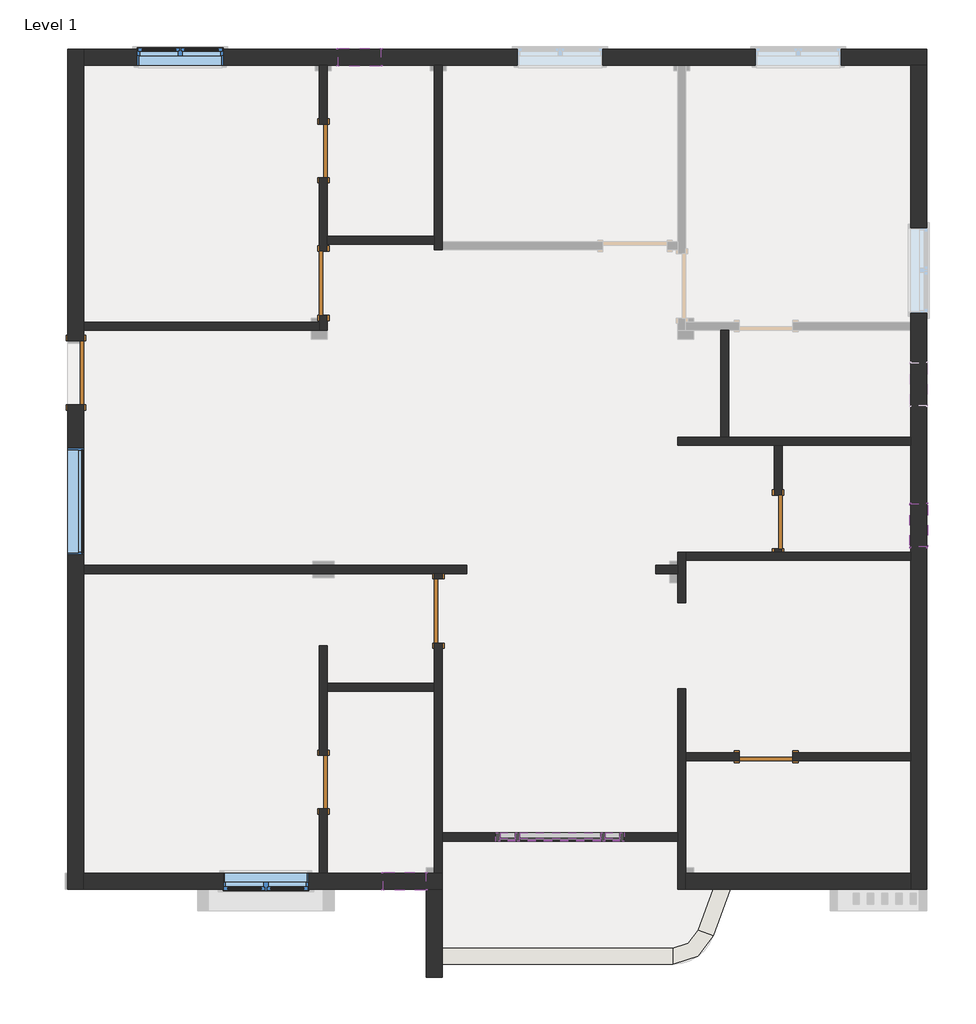
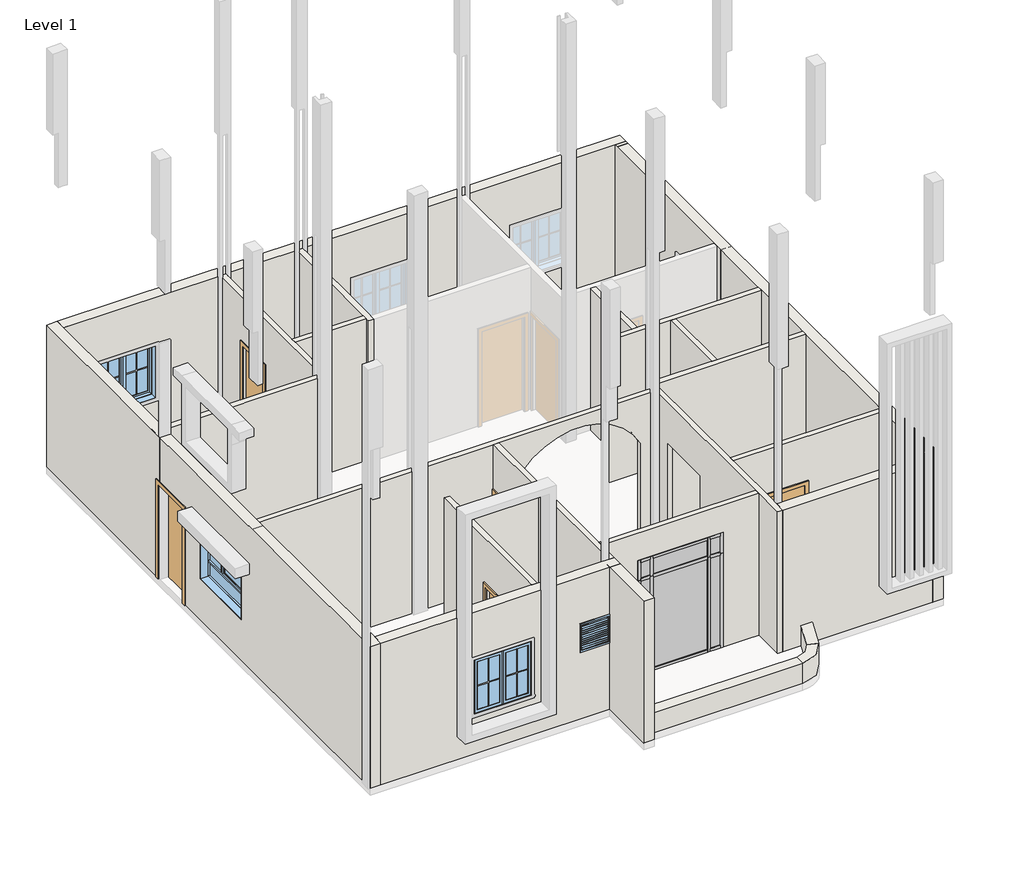
# One storey, part 1 of 2: 24 walls, 17 members, 7 doors, 6 plates, 6 windows.
"""IFC4 building model written with IfcOpenShell, lengths in millimetres."""

from ifc_helpers import new_model, si_unit, point, frame, frame_2d, origin, origin_with_axes, place, context, project, spatial, polyline, circle_curve, trimmed, segment, composite_curve, outline, extrude, faceted_brep, transform, mapped, element, save
from ifc_brep_helpers import plane_surface, revolved_surface, advanced_brep
from components import door_78caadf7, door_214872d5, door_305aa2a5, door_e5f9f3c4, door_a90ba1ad, member_420b45ef, member_7cbddb58, member_a5966c2a, member_0585f7b2, member_d7472725, member_ffd4c858, member_15823cb3, member_3374d9b6, system_panel_glazed_ab75977c, system_panel_glazed_55699693, system_panel_glazed_94a389e0, system_panel_glazed_496eb5f8, window_awning_variable_5_x4_e7258766, window_af3140d2, window_f2d8fef0

model = new_model("IFC4")

# Units and contexts
model_context = context("Model", 3, world=origin())
ifc_project = project(units=[si_unit("LENGTHUNIT", "METRE", prefix="MILLI")], contexts=[model_context])

# Site, building, storey
site = spatial("IfcSite", under=ifc_project)
building = spatial("IfcBuilding", under=site)
storey = spatial("IfcBuildingStorey", under=building, Name="Level 1", Elevation=0.0)

# Doors
placement = place(None, origin())
door_shape = door_78caadf7(model_context)
element("IfcDoor", 1, ObjectType="Single-Flush : 2'6\"x 7'", at=placement, inside=storey, context=model_context, shape_type="MappedRepresentation", body=[
    mapped(door_shape, transform((-11257.4178125, 12083.816018, 0.0), x_axis=(0.0, 1.0, 0.0), y_axis=(-1.0, 0.0, 0.0), z_axis=(0.0, 0.0, 1.0))),
])
element("IfcDoor", 2, ObjectType="Single-Flush : 2'6\"x 7'", at=placement, inside=storey, context=model_context, shape_type="MappedRepresentation", body=[
    mapped(door_shape, transform((-11257.4178125, 3092.216018, 0.0), x_axis=(0.0, 1.0, 0.0), y_axis=(-1.0, 0.0, 0.0), z_axis=(0.0, 0.0, 1.0))),
])
door_2_shape = door_214872d5(model_context)
element("IfcDoor", 3, ObjectType="Single-Flush : 2'6\"x 7'", at=placement, inside=storey, context=model_context, shape_type="MappedRepresentation", body=[
    mapped(door_2_shape, transform((-4780.4178125, 6800.616018, 0.0), x_axis=(0.0, -1.0, 0.0), y_axis=(1.0, 0.0, 0.0), z_axis=(0.0, 0.0, 1.0))),
])
element("IfcDoor", 4, ObjectType="Single-Flush : 2'6\"x 7'", at=placement, inside=storey, context=model_context, shape_type="MappedRepresentation", body=[
    mapped(door_2_shape, transform((-4951.8678125, 3454.166018, 0.0), x_axis=(-1.0, 0.0, 0.0), y_axis=(0.0, -1.0, 0.0), z_axis=(0.0, 0.0, 1.0))),
])
door_3_shape = door_305aa2a5(model_context)
element("IfcDoor", 5, ObjectType="Single-Flush : 36\" x 84\"", at=placement, inside=storey, context=model_context, shape_type="MappedRepresentation", body=[
    mapped(door_3_shape, transform((-11257.4178125, 10197.866018, 0.0), x_axis=(0.0, -1.0, 0.0), y_axis=(1.0, 0.0, 0.0), z_axis=(0.0, 0.0, 1.0))),
])
door_4_shape = door_e5f9f3c4(model_context)
element("IfcDoor", 6, ObjectType="Single-Flush : 36\" x 84\"", at=placement, inside=storey, context=model_context, shape_type="MappedRepresentation", body=[
    mapped(door_4_shape, transform((-9619.1178125, 5530.616018, 0.0), x_axis=(0.0, 1.0, 0.0), y_axis=(-1.0, 0.0, 0.0), z_axis=(0.0, 0.0, 1.0))),
])
door_5_shape = door_a90ba1ad(model_context)
element("IfcDoor", 7, ObjectType="Single-Flush : 36\" x 84\"", at=placement, inside=storey, context=model_context, shape_type="MappedRepresentation", body=[
    mapped(door_5_shape, transform((-14781.6678125, 8921.516018, 0.0), x_axis=(0.0, 1.0, 0.0), y_axis=(-1.0, 0.0, 0.0), z_axis=(0.0, 0.0, 1.0))),
])

# Members
member_shape = member_420b45ef(model_context)
element("IfcMember", 8, ObjectType="Rectangular Mullion : 2.5\" x 5\" rectangular", at=placement, inside=storey, context=model_context, shape_type="MappedRepresentation", body=[
    mapped(member_shape, transform((-8736.4678125, 2311.166018, 2590.8), x_axis=(0.0, 0.0, 1.0), y_axis=(0.0, 1.0, 0.0), z_axis=(-1.0, 0.0, 0.0))),
])
element("IfcMember", 9, ObjectType="Rectangular Mullion : 2.5\" x 5\" rectangular", at=placement, inside=storey, context=model_context, shape_type="MappedRepresentation", body=[
    mapped(member_shape, transform((-7244.2178125, 2311.166018, 2590.8), x_axis=(0.0, 0.0, 1.0), y_axis=(0.0, 1.0, 0.0), z_axis=(-1.0, 0.0, 0.0))),
])
element("IfcMember", 10, ObjectType="Rectangular Mullion : 2.5\" x 5\" rectangular", at=placement, inside=storey, context=model_context, shape_type="MappedRepresentation", body=[
    mapped(member_shape, transform((-7034.6678125, 2311.166018, 0.0), x_axis=(0.0, 0.0, -1.0), y_axis=(0.0, 1.0, 0.0), z_axis=(1.0, 0.0, 0.0))),
])
element("IfcMember", 11, ObjectType="Rectangular Mullion : 2.5\" x 5\" rectangular", at=placement, inside=storey, context=model_context, shape_type="MappedRepresentation", body=[
    mapped(member_shape, transform((-8526.9178125, 2311.166018, 0.0), x_axis=(0.0, 0.0, -1.0), y_axis=(0.0, 1.0, 0.0), z_axis=(1.0, 0.0, 0.0))),
])
member_2_shape = member_7cbddb58(model_context)
element("IfcMember", 12, ObjectType="Rectangular Mullion : 2.5\" x 5\" rectangular", at=placement, inside=storey, context=model_context, shape_type="MappedRepresentation", body=[
    mapped(member_2_shape, transform((-7275.9678125, 2311.166018, 0.0), x_axis=(-1.0, 0.0, 0.0), y_axis=(0.0, 1.0, 0.0), z_axis=(0.0, 0.0, -1.0))),
])
element("IfcMember", 13, ObjectType="Rectangular Mullion : 2.5\" x 5\" rectangular", at=placement, inside=storey, context=model_context, shape_type="MappedRepresentation", body=[
    mapped(member_2_shape, transform((-8495.1678125, 2311.166018, 0.0), x_axis=(-1.0, 0.0, 0.0), y_axis=(0.0, 1.0, 0.0), z_axis=(0.0, 0.0, -1.0))),
])
member_3_shape = member_a5966c2a(model_context)
element("IfcMember", 14, ObjectType="Rectangular Mullion : 2.5\" x 5\" rectangular", at=placement, inside=storey, context=model_context, shape_type="MappedRepresentation", body=[
    mapped(member_3_shape, transform((-7244.2178125, 2311.166018, 2133.6), x_axis=(0.0, 0.0, 1.0), y_axis=(0.0, 1.0, 0.0), z_axis=(-1.0, 0.0, 0.0))),
])
element("IfcMember", 15, ObjectType="Rectangular Mullion : 2.5\" x 5\" rectangular", at=placement, inside=storey, context=model_context, shape_type="MappedRepresentation", body=[
    mapped(member_3_shape, transform((-8736.4678125, 2311.166018, 2133.6), x_axis=(0.0, 0.0, 1.0), y_axis=(0.0, 1.0, 0.0), z_axis=(-1.0, 0.0, 0.0))),
])
member_4_shape = member_0585f7b2(model_context)
element("IfcMember", 16, ObjectType="Rectangular Mullion : 2.5\" x 5\" rectangular", at=placement, inside=storey, context=model_context, shape_type="MappedRepresentation", body=[
    mapped(member_4_shape, transform((-8463.4178125, 2311.166018, 2133.6), x_axis=(0.0, 0.0, 1.0), y_axis=(0.0, 1.0, 0.0), z_axis=(-1.0, 0.0, 0.0))),
])
member_5_shape = member_d7472725(model_context)
element("IfcMember", 17, ObjectType="Rectangular Mullion : 2.5\" x 5\" rectangular", at=placement, inside=storey, context=model_context, shape_type="MappedRepresentation", body=[
    mapped(member_5_shape, transform((-7307.7178125, 2311.166018, 0.0), x_axis=(0.0, 0.0, -1.0), y_axis=(0.0, 1.0, 0.0), z_axis=(1.0, 0.0, 0.0))),
])
element("IfcMember", 18, ObjectType="Rectangular Mullion : 2.5\" x 5\" rectangular", at=placement, inside=storey, context=model_context, shape_type="MappedRepresentation", body=[
    mapped(member_5_shape, transform((-8463.4178125, 2311.166018, 2590.8), x_axis=(0.0, 0.0, 1.0), y_axis=(0.0, 1.0, 0.0), z_axis=(-1.0, 0.0, 0.0))),
])
member_6_shape = member_ffd4c858(model_context)
element("IfcMember", 19, ObjectType="Rectangular Mullion : 2.5\" x 5\" rectangular", at=placement, inside=storey, context=model_context, shape_type="MappedRepresentation", body=[
    mapped(member_6_shape, transform((-7275.9678125, 2311.166018, 2133.6), x_axis=(-1.0, 0.0, 0.0), y_axis=(0.0, 1.0, 0.0), z_axis=(0.0, 0.0, -1.0))),
])
element("IfcMember", 20, ObjectType="Rectangular Mullion : 2.5\" x 5\" rectangular", at=placement, inside=storey, context=model_context, shape_type="MappedRepresentation", body=[
    mapped(member_6_shape, transform((-8495.1678125, 2311.166018, 2133.6), x_axis=(-1.0, 0.0, 0.0), y_axis=(0.0, 1.0, 0.0), z_axis=(0.0, 0.0, -1.0))),
])
member_7_shape = member_15823cb3(model_context)
element("IfcMember", 21, ObjectType="Rectangular Mullion : 2.5\" x 5\" rectangular", at=placement, inside=storey, context=model_context, shape_type="MappedRepresentation", body=[
    mapped(member_7_shape, transform((-6971.1678125, 2311.166018, 2590.8), x_axis=(1.0, 0.0, 0.0), y_axis=(0.0, 1.0, 0.0), z_axis=(0.0, 0.0, 1.0))),
])
member_8_shape = member_3374d9b6(model_context)
element("IfcMember", 22, ObjectType="Rectangular Mullion : 2.5\" x 5\" rectangular", at=placement, inside=storey, context=model_context, shape_type="MappedRepresentation", body=[
    mapped(member_8_shape, transform((-8799.9678125, 2311.166018, 0.0), x_axis=(-1.0, 0.0, 0.0), y_axis=(0.0, 1.0, 0.0), z_axis=(0.0, 0.0, -1.0))),
])
element("IfcMember", 23, ObjectType="Rectangular Mullion : 2.5\" x 5\" rectangular", at=placement, inside=storey, context=model_context, shape_type="MappedRepresentation", body=[
    mapped(member_7_shape, transform((-8799.9678125, 2311.166018, 2133.6), x_axis=(-1.0, 0.0, 0.0), y_axis=(0.0, 1.0, 0.0), z_axis=(0.0, 0.0, -1.0))),
])
element("IfcMember", 24, ObjectType="Rectangular Mullion : 2.5\" x 5\" rectangular", at=placement, inside=storey, context=model_context, shape_type="MappedRepresentation", body=[
    mapped(member_8_shape, transform((-6971.1678125, 2311.166018, 2133.6), x_axis=(1.0, 0.0, 0.0), y_axis=(0.0, 1.0, 0.0), z_axis=(0.0, 0.0, 1.0))),
])

# Plates
system_panel_glazed_shape = system_panel_glazed_ab75977c(model_context)
element("IfcPlate", 25, ObjectType="System Panel : Glazed", at=placement, inside=storey, context=model_context, shape_type="MappedRepresentation", body=[
    mapped(system_panel_glazed_shape, transform((-7139.4428125, 2311.166018, 63.5), x_axis=(-1.0, 0.0, 0.0), y_axis=(0.0, -1.0, 0.0), z_axis=(0.0, 0.0, 1.0))),
])
element("IfcPlate", 26, ObjectType="System Panel : Glazed", at=placement, inside=storey, context=model_context, shape_type="MappedRepresentation", body=[
    mapped(system_panel_glazed_shape, transform((-8631.6928125, 2311.166018, 63.5), x_axis=(-1.0, 0.0, 0.0), y_axis=(0.0, -1.0, 0.0), z_axis=(0.0, 0.0, 1.0))),
])
system_panel_glazed_2_shape = system_panel_glazed_55699693(model_context)
element("IfcPlate", 27, ObjectType="System Panel : Glazed", at=placement, inside=storey, context=model_context, shape_type="MappedRepresentation", body=[
    mapped(system_panel_glazed_2_shape, transform((-7885.5678125, 2311.166018, 63.5), x_axis=(-1.0, 0.0, 0.0), y_axis=(0.0, -1.0, 0.0), z_axis=(0.0, 0.0, 1.0))),
])
system_panel_glazed_3_shape = system_panel_glazed_94a389e0(model_context)
element("IfcPlate", 28, ObjectType="System Panel : Glazed", at=placement, inside=storey, context=model_context, shape_type="MappedRepresentation", body=[
    mapped(system_panel_glazed_3_shape, transform((-7139.4428125, 2311.166018, 2165.35), x_axis=(-1.0, 0.0, 0.0), y_axis=(0.0, -1.0, 0.0), z_axis=(0.0, 0.0, 1.0))),
])
element("IfcPlate", 29, ObjectType="System Panel : Glazed", at=placement, inside=storey, context=model_context, shape_type="MappedRepresentation", body=[
    mapped(system_panel_glazed_3_shape, transform((-8631.6928125, 2311.166018, 2165.35), x_axis=(-1.0, 0.0, 0.0), y_axis=(0.0, -1.0, 0.0), z_axis=(0.0, 0.0, 1.0))),
])
system_panel_glazed_4_shape = system_panel_glazed_496eb5f8(model_context)
element("IfcPlate", 30, ObjectType="System Panel : Glazed", at=placement, inside=storey, context=model_context, shape_type="MappedRepresentation", body=[
    mapped(system_panel_glazed_4_shape, transform((-7885.5678125, 2311.166018, 2165.35), x_axis=(-1.0, 0.0, 0.0), y_axis=(0.0, -1.0, 0.0), z_axis=(0.0, 0.0, 1.0))),
])

# Walls
element("IfcWall", 31, ObjectType="4.5\" wall", at=placement, inside=storey, context=model_context, shape_type="Brep", body=[
    faceted_brep([(-11314.5678125, 9740.666018, 2133.6), (-11314.5678125, 9740.666018, 0.0), (-11314.5678125, 9702.566018, 0.0), (-11314.5678125, 9645.416018, 0.0), (-11314.5678125, 9531.116018, 0.0), (-11314.5678125, 9531.116018, 3200.4), (-11314.5678125, 9645.416018, 3200.4), (-11314.5678125, 13303.016018, 3200.4), (-11314.5678125, 13303.016018, 0.0), (-11314.5678125, 13226.816018, 0.0), (-11314.5678125, 12464.816018, 0.0), (-11314.5678125, 12464.816018, 2133.6), (-11314.5678125, 11702.816018, 2133.6), (-11314.5678125, 11702.816018, 0.0), (-11314.5678125, 10655.066018, 0.0), (-11314.5678125, 10655.066018, 2133.6), (-11200.2678125, 9531.116018, 0.0), (-11200.2678125, 9740.666018, 0.0), (-11200.2678125, 9740.666018, 2133.6), (-11200.2678125, 10655.066018, 2133.6), (-11200.2678125, 10655.066018, 0.0), (-11200.2678125, 10750.316018, 0.0), (-11200.2678125, 10864.616018, 0.0), (-11200.2678125, 11702.816018, 0.0), (-11200.2678125, 11702.816018, 2133.6), (-11200.2678125, 12464.816018, 2133.6), (-11200.2678125, 12464.816018, 0.0), (-11200.2678125, 13226.816018, 0.0), (-11200.2678125, 13303.016018, 0.0), (-11200.2678125, 13303.016018, 3200.4), (-11200.2678125, 10864.616018, 3200.4), (-11200.2678125, 10750.316018, 3200.4), (-11200.2678125, 9531.116018, 3200.4)], [[[0, 1, 2, 3, 4, 5, 6, 7, 8, 9, 10, 11, 12, 13, 14, 15]], [[16, 17, 18, 19, 20, 21, 22, 23, 24, 25, 26, 27, 28, 29, 30, 31, 32]], [[14, 13, 23, 22, 21, 20]], [[4, 3, 2, 1, 17, 16]], [[28, 27, 26, 10, 9, 8]], [[7, 6, 5, 32, 31, 30, 29]], [[8, 7, 29, 28]], [[5, 4, 16, 32]], [[11, 10, 26, 25]], [[12, 11, 25, 24]], [[13, 12, 24, 23]], [[18, 17, 1, 0]], [[19, 18, 0, 15]], [[20, 19, 15, 14]]]),
])
element("IfcWall", 32, ObjectType="4.5\" wall", at=placement, inside=storey, context=model_context, shape_type="Brep", body=[
    faceted_brep([(-14667.3678125, 9531.116018, 0.0), (-11428.8678125, 9531.116018, 0.0), (-11314.5678125, 9531.116018, 0.0), (-11314.5678125, 9531.116018, 3200.4), (-14667.3678125, 9531.116018, 3200.4), (-14667.3678125, 9645.416018, 0.0), (-14667.3678125, 9645.416018, 3200.4), (-11314.5678125, 9645.416018, 3200.4), (-11314.5678125, 9645.416018, 0.0), (-11428.8678125, 9645.416018, 0.0)], [[[0, 1, 2, 3, 4]], [[5, 6, 7, 8, 9]], [[2, 1, 0, 5, 9, 8]], [[4, 3, 7, 6]], [[0, 4, 6, 5]], [[3, 2, 8, 7]]]),
])
element("IfcWall", 33, ObjectType="4.5\" wall", at=placement, inside=storey, context=model_context, shape_type="Brep", body=[
    faceted_brep([(-9676.2678125, 13303.016018, 0.0), (-9676.2678125, 13226.816018, 0.0), (-9676.2678125, 10864.616018, 0.0), (-9676.2678125, 10750.316018, 0.0), (-9676.2678125, 10674.116018, 0.0), (-9676.2678125, 10674.116018, 3200.4), (-9676.2678125, 10750.316018, 3200.4), (-9676.2678125, 10864.616018, 3200.4), (-9676.2678125, 13303.016018, 3200.4), (-9561.9678125, 13303.016018, 0.0), (-9561.9678125, 13303.016018, 3200.4), (-9561.9678125, 10788.416018, 3200.4), (-9561.9678125, 10674.116018, 3200.4), (-9561.9678125, 10674.116018, 0.0), (-9561.9678125, 10788.416018, 0.0), (-9561.9678125, 13226.816018, 0.0)], [[[0, 1, 2, 3, 4, 5, 6, 7, 8]], [[9, 10, 11, 12, 13, 14, 15]], [[4, 3, 2, 1, 0, 9, 15, 14, 13]], [[8, 7, 6, 5, 12, 11, 10]], [[0, 8, 10, 9]], [[5, 4, 13, 12]]]),
])
element("IfcWall", 34, ObjectType="4.5\" wall", at=placement, inside=storey, context=model_context, shape_type="SweptSolid", body=[
    extrude(outline(polyline([(-9676.2678125, 10750.316018), (-11200.2678125, 10750.316018), (-11200.2678125, 10864.616018), (-9676.2678125, 10864.616018), (-9676.2678125, 10750.316018)])), origin_with_axes(), (0.0, 0.0, 1.0), 3200.4),
])
element("IfcWall", 35, ObjectType="4.5\" wall", at=placement, inside=storey, context=model_context, shape_type="AdvancedBrep", body=[
    advanced_brep(
    [(-14667.3678125, 6064.016018, 0.0), (-11409.8178125, 6064.016018, 0.0), (-11105.0178125, 6064.016018, 0.0), (-9676.2678125, 6064.016018, 0.0), (-9561.9678125, 6064.016018, 0.0), (-9216.6666467, 6064.016018, 0.0), (-9216.6666467, 6064.016018, 2133.6), (-6524.2666467, 6064.016018, 2133.6), (-6524.2666467, 6064.016018, 0.0), (-6323.4678125, 6064.016018, 0.0), (-6209.1678125, 6064.016018, 0.0), (-6209.1678125, 6064.016018, 3200.4), (-9561.9678125, 6064.016018, 3200.4), (-9676.2678125, 6064.016018, 3200.4), (-14667.3678125, 6064.016018, 3200.4), (-14667.3678125, 6178.316018, 0.0), (-14667.3678125, 6178.316018, 3200.4), (-6209.1678125, 6178.316018, 3200.4), (-6209.1678125, 6178.316018, 0.0), (-6323.4678125, 6178.316018, 0.0), (-6524.2666467, 6178.316018, 0.0), (-6524.2666467, 6178.316018, 2133.6), (-9216.6666467, 6178.316018, 2133.6), (-9216.6666467, 6178.316018, 0.0), (-11105.0178125, 6178.316018, 0.0), (-11409.8178125, 6178.316018, 0.0)],
    [
        (0, 1),
        (1, 2),
        (2, 3),
        (3, 4),
        (4, 5),
        (5, 6),
        (6, 7, circle_curve(frame((-7870.4666467, 6064.016018, 1433.7183788), z_axis=(0.0, 1.0, 0.0), x_axis=(-1.0, 0.0, 0.0)), 1517.2635644)),
        (7, 8),
        (8, 9),
        (9, 10),
        (10, 11),
        (11, 12),
        (12, 13),
        (13, 14),
        (14, 0),
        (15, 16),
        (16, 17),
        (17, 18),
        (18, 19),
        (19, 20),
        (20, 21),
        (21, 22, circle_curve(frame((-7870.4666467, 6178.316018, 1433.7183788), z_axis=(0.0, -1.0, 0.0), x_axis=(-1.0, 0.0, 0.0)), 1517.2635644)),
        (22, 23),
        (23, 24),
        (24, 25),
        (25, 15),
        (14, 16),
        (15, 0),
        (10, 18),
        (17, 11),
        (23, 5),
        (22, 6),
        (21, 7),
        (20, 8),
    ],
    [
        plane_surface(frame((-3919.5354576, 6064.016018, 0.0), z_axis=(0.0, -1.0, 0.0), x_axis=(1.0, 0.0, 0.0))),
        plane_surface(frame((-3919.5354576, 6178.316018, 0.0), z_axis=(0.0, 1.0, 0.0), x_axis=(-1.0, 0.0, 0.0))),
        plane_surface(frame((-14667.3678125, 13531.616018, 0.0), z_axis=(-1.0, 0.0, 0.0), x_axis=(0.0, 1.0, 0.0))),
        plane_surface(frame((-6209.1678125, 6010.7399841, 0.0), z_axis=(1.0, 0.0, 0.0), x_axis=(0.0, -1.0, 0.0))),
        plane_surface(frame((-14781.6678125, 6064.016018, 0.0), z_axis=(0.0, 0.0, -1.0), x_axis=(0.0, 1.0, 0.0))),
        plane_surface(frame((-6152.0178125, 6064.016018, 3200.4), z_axis=(0.0, 0.0, 1.0), x_axis=(0.0, 1.0, 0.0))),
        plane_surface(frame((-9216.6666467, 6064.016018, 0.0), z_axis=(1.0, 0.0, 0.0), x_axis=(0.0, 1.0, 0.0))),
        revolved_surface(polyline([(-9387.730211099999, 6178.316018, 1433.7183788), (-9387.730211099999, 6064.016018, 1433.7183788)]), (-7870.4666467, 6178.316018, 1433.7183788), (0.0, 1.0, 0.0)),
        plane_surface(frame((-6524.2666467, 6064.016018, 2133.6), z_axis=(-1.0, 0.0, 0.0), x_axis=(0.0, 1.0, 0.0))),
        plane_surface(frame((-6524.2666467, 6064.016018, 0.0), z_axis=(0.0, 0.0, -1.0), x_axis=(0.0, 1.0, 0.0))),
    ],
    [
        (0, [[1, 2, 3, 4, 5, 6, 7, 8, 9, 10, 11, 12, 13, 14, 15]]),
        (1, [[16, 17, 18, 19, 20, 21, 22, 23, 24, 25, 26]]),
        (2, [[-15, 27, -16, 28]]),
        (3, [[-11, 29, -18, 30]]),
        (4, [[-5, -4, -3, -2, -1, -28, -26, -25, -24, 31]]),
        (5, [[-14, -13, -12, -30, -17, -27]]),
        (6, [[-6, -31, -23, 32]]),
        (7, [[-7, -32, -22, 33]]),
        (8, [[-8, -33, -21, 34]]),
        (9, [[-10, -9, -34, -20, -19, -29]]),
    ],
),
])
element("IfcWall", 36, ObjectType="4.5\" wall", at=placement, inside=storey, context=model_context, shape_type="Brep", body=[
    faceted_brep([(-11314.5678125, 5035.316018, 0.0), (-11314.5678125, 3473.216018, 0.0), (-11314.5678125, 3473.216018, 2133.6), (-11314.5678125, 2711.216018, 2133.6), (-11314.5678125, 2711.216018, 0.0), (-11314.5678125, 1796.816018, 0.0), (-11314.5678125, 1796.816018, 3200.4), (-11314.5678125, 5035.316018, 3200.4), (-11200.2678125, 3473.216018, 2133.6), (-11200.2678125, 3473.216018, 0.0), (-11200.2678125, 4387.616018, 0.0), (-11200.2678125, 4501.916018, 0.0), (-11200.2678125, 5035.316018, 0.0), (-11200.2678125, 5035.316018, 3200.4), (-11200.2678125, 4501.916018, 3200.4), (-11200.2678125, 4387.616018, 3200.4), (-11200.2678125, 1796.816018, 3200.4), (-11200.2678125, 1796.816018, 0.0), (-11200.2678125, 2711.216018, 0.0), (-11200.2678125, 2711.216018, 2133.6)], [[[0, 1, 2, 3, 4, 5, 6, 7]], [[8, 9, 10, 11, 12, 13, 14, 15, 16, 17, 18, 19]], [[18, 17, 5, 4]], [[12, 11, 10, 9, 1, 0]], [[7, 6, 16, 15, 14, 13]], [[0, 7, 13, 12]], [[6, 5, 17, 16]], [[2, 1, 9, 8]], [[3, 2, 8, 19]], [[4, 3, 19, 18]]]),
])
element("IfcWall", 37, ObjectType="4.5\" wall", at=placement, inside=storey, context=model_context, shape_type="Brep", body=[
    faceted_brep([(-9561.9678125, 5987.816018, 2133.6), (-9561.9678125, 5987.816018, 0.0), (-9561.9678125, 6064.016018, 0.0), (-9561.9678125, 6064.016018, 3200.4), (-9561.9678125, 2368.316018, 3200.4), (-9561.9678125, 2254.016018, 3200.4), (-9561.9678125, 1796.816018, 3200.4), (-9561.9678125, 1796.816018, 0.0), (-9561.9678125, 2254.016018, 0.0), (-9561.9678125, 2368.316018, 0.0), (-9561.9678125, 5073.416018, 0.0), (-9561.9678125, 5073.416018, 2133.6), (-9676.2678125, 6064.016018, 0.0), (-9676.2678125, 5987.816018, 0.0), (-9676.2678125, 5987.816018, 2133.6), (-9676.2678125, 5073.416018, 2133.6), (-9676.2678125, 5073.416018, 0.0), (-9676.2678125, 4501.916018, 0.0), (-9676.2678125, 4387.616018, 0.0), (-9676.2678125, 1873.016018, 0.0), (-9676.2678125, 1796.816018, 0.0), (-9676.2678125, 1796.816018, 3200.4), (-9676.2678125, 4387.616018, 3200.4), (-9676.2678125, 4501.916018, 3200.4), (-9676.2678125, 6064.016018, 3200.4)], [[[0, 1, 2, 3, 4, 5, 6, 7, 8, 9, 10, 11]], [[12, 13, 14, 15, 16, 17, 18, 19, 20, 21, 22, 23, 24]], [[2, 1, 13, 12]], [[10, 9, 8, 7, 20, 19, 18, 17, 16]], [[6, 5, 4, 3, 24, 23, 22, 21]], [[7, 6, 21, 20]], [[14, 13, 1, 0]], [[15, 14, 0, 11]], [[16, 15, 11, 10]], [[3, 2, 12, 24]]]),
])
element("IfcWall", 38, ObjectType="4.5\" wall", at=placement, inside=storey, context=model_context, shape_type="SweptSolid", body=[
    extrude(outline(polyline([(-9676.2678125, 4387.616018), (-11200.2678125, 4387.616018), (-11200.2678125, 4501.916018), (-9676.2678125, 4501.916018), (-9676.2678125, 4387.616018)])), origin_with_axes(), (0.0, 0.0, 1.0), 3200.4),
])
element("IfcWall", 39, ObjectType="4.5\" wall", at=placement, inside=storey, context=model_context, shape_type="Brep", body=[
    faceted_brep([(-6094.8678125, 6368.816018, 0.0), (-6094.8678125, 6368.816018, 3200.4), (-6094.8678125, 6254.516018, 3200.4), (-6094.8678125, 3511.316018, 3200.4), (-6094.8678125, 3397.016018, 3200.4), (-6094.8678125, 1796.816018, 3200.4), (-6094.8678125, 1568.216018, 3200.4), (-6094.8678125, 1568.216018, 0.0), (-6094.8678125, 1796.816018, 0.0), (-6094.8678125, 1873.016018, 0.0), (-6094.8678125, 3397.016018, 0.0), (-6094.8678125, 3511.316018, 0.0), (-6094.8678125, 4425.716018, 0.0), (-6094.8678125, 4425.716018, 2286.0), (-6094.8678125, 5644.916018, 2286.0), (-6094.8678125, 5644.916018, 0.0), (-6094.8678125, 6254.516018, 0.0), (-6209.1678125, 6368.816018, 3200.4), (-6209.1678125, 6368.816018, 0.0), (-6209.1678125, 6235.466018, 0.0), (-6209.1678125, 6178.316018, 0.0), (-6209.1678125, 6064.016018, 0.0), (-6209.1678125, 5930.666018, 0.0), (-6209.1678125, 5644.916018, 0.0), (-6209.1678125, 5644.916018, 2286.0), (-6209.1678125, 4425.716018, 2286.0), (-6209.1678125, 4425.716018, 0.0), (-6209.1678125, 2368.316018, 0.0), (-6209.1678125, 2254.016018, 0.0), (-6209.1678125, 1568.216018, 0.0), (-6209.1678125, 1568.216018, 3200.4), (-6209.1678125, 2254.016018, 3200.4), (-6209.1678125, 2368.316018, 3200.4), (-6209.1678125, 6064.016018, 3200.4), (-6209.1678125, 6178.316018, 3200.4)], [[[0, 1, 2, 3, 4, 5, 6, 7, 8, 9, 10, 11, 12, 13, 14, 15, 16]], [[17, 18, 19, 20, 21, 22, 23, 24, 25, 26, 27, 28, 29, 30, 31, 32, 33, 34]], [[18, 0, 16, 15, 23, 22, 21, 20, 19]], [[7, 29, 28, 27, 26, 12, 11, 10, 9, 8]], [[6, 5, 4, 3, 2, 1, 17, 34, 33, 32, 31, 30]], [[1, 0, 18, 17]], [[7, 6, 30, 29]], [[13, 25, 24, 14]], [[25, 13, 12, 26]], [[14, 24, 23, 15]]]),
])
element("IfcWall", 40, ObjectType="4.5\" wall", at=placement, inside=storey, context=model_context, shape_type="Brep", body=[
    faceted_brep([(-2894.4678125, 8007.116018, 0.0), (-5485.2678125, 8007.116018, 0.0), (-5599.5678125, 8007.116018, 0.0), (-6209.1678125, 8007.116018, 0.0), (-6209.1678125, 8007.116018, 3200.4), (-5599.5678125, 8007.116018, 3200.4), (-5485.2678125, 8007.116018, 3200.4), (-2894.4678125, 8007.116018, 3200.4), (-2894.4678125, 7892.816018, 0.0), (-2894.4678125, 7892.816018, 3200.4), (-4723.2678125, 7892.816018, 3200.4), (-4837.5678125, 7892.816018, 3200.4), (-6209.1678125, 7892.816018, 3200.4), (-6209.1678125, 7892.816018, 0.0), (-4837.5678125, 7892.816018, 0.0), (-4723.2678125, 7892.816018, 0.0)], [[[0, 1, 2, 3, 4, 5, 6, 7]], [[8, 9, 10, 11, 12, 13, 14, 15]], [[3, 2, 1, 0, 8, 15, 14, 13]], [[4, 3, 13, 12]], [[7, 6, 5, 4, 12, 11, 10, 9]], [[0, 7, 9, 8]]]),
])
element("IfcWall", 41, ObjectType="4.5\" wall", at=placement, inside=storey, context=model_context, shape_type="Brep", body=[
    faceted_brep([(-2894.4678125, 6368.816018, 0.0), (-4723.2678125, 6368.816018, 0.0), (-4837.5678125, 6368.816018, 0.0), (-6094.8678125, 6368.816018, 0.0), (-6094.8678125, 6368.816018, 3200.4), (-4837.5678125, 6368.816018, 3200.4), (-4723.2678125, 6368.816018, 3200.4), (-2894.4678125, 6368.816018, 3200.4), (-2894.4678125, 6254.516018, 0.0), (-2894.4678125, 6254.516018, 3200.4), (-6094.8678125, 6254.516018, 3200.4), (-6094.8678125, 6254.516018, 0.0)], [[[0, 1, 2, 3, 4, 5, 6, 7]], [[8, 9, 10, 11]], [[3, 2, 1, 0, 8, 11]], [[7, 6, 5, 4, 10, 9]], [[0, 7, 9, 8]], [[4, 3, 11, 10]]]),
])
element("IfcWall", 42, ObjectType="4.5\" wall", at=placement, inside=storey, context=model_context, shape_type="SweptSolid", body=[
    extrude(outline(polyline([(0.0, -6094.8678125), (0.0, -5332.8678125), (2133.6, -5332.8678125), (2133.6, -4570.8678125), (0.0, -4570.8678125), (0.0, -2894.4678125), (3200.4, -2894.4678125), (3200.4, -6094.8678125), (0.0, -6094.8678125)])), frame((0.0, 3397.016018, 0.0), z_axis=(0.0, 1.0, 0.0), x_axis=(0.0, 0.0, 1.0)), (0.0, 0.0, 1.0), 114.3),
])
element("IfcWall", 43, ObjectType="4.5\" wall", at=placement, inside=storey, context=model_context, shape_type="SweptSolid", body=[
    extrude(outline(polyline([(-5599.5678125, 8007.116018), (-5599.5678125, 9531.116018), (-5485.2678125, 9531.116018), (-5485.2678125, 8007.116018), (-5599.5678125, 8007.116018)])), origin_with_axes(), (0.0, 0.0, 1.0), 3200.4),
])
element("IfcWall", 44, ObjectType="4.5\" wall", at=placement, inside=storey, context=model_context, shape_type="SweptSolid", body=[
    extrude(outline(polyline([(6419.616018, 2133.6), (6419.616018, 0.0), (6368.816018, 0.0), (6368.816018, 3200.4), (7892.816018, 3200.4), (7892.816018, 0.0), (7181.616018, 0.0), (7181.616018, 2133.6), (6419.616018, 2133.6)])), frame((-4837.5678125, 0.0, 0.0), z_axis=(1.0, 0.0, 0.0), x_axis=(0.0, 1.0, 0.0)), (0.0, 0.0, 1.0), 114.3),
])
element("IfcWall", 45, ObjectType="4.5\" wall", at=placement, inside=storey, context=model_context, shape_type="SweptSolid", body=[
    extrude(outline(polyline([(3200.4, -6209.1678125), (3200.4, -9561.9678125), (0.0, -9561.9678125), (0.0, -8799.9678125), (2590.8, -8799.9678125), (2590.8, -6971.1678125), (0.0, -6971.1678125), (0.0, -6209.1678125), (3200.4, -6209.1678125)])), frame((0.0, 2254.016018, 0.0), z_axis=(0.0, 1.0, 0.0), x_axis=(0.0, 0.0, 1.0)), (0.0, 0.0, 1.0), 114.3),
])
element("IfcWall", 46, ObjectType="9\" wall", at=placement, inside=storey, context=model_context, shape_type="Brep", body=[
    faceted_brep([(-14895.9678125, 13531.616018, 0.0), (-14895.9678125, 9378.716018, 0.0), (-14895.9678125, 9378.716018, 2133.6), (-14895.9678125, 8464.316018, 2133.6), (-14895.9678125, 8464.316018, 0.0), (-14895.9678125, 1796.816018, 0.0), (-14895.9678125, 1568.216018, 0.0), (-14895.9678125, 1568.216018, 3200.4), (-14895.9678125, 13531.616018, 3200.4), (-14895.9678125, 6330.716018, 2133.6), (-14895.9678125, 6330.716018, 914.4), (-14895.9678125, 7854.716018, 914.4), (-14895.9678125, 7854.716018, 2133.6), (-14667.3678125, 9378.716018, 2133.6), (-14667.3678125, 9378.716018, 0.0), (-14667.3678125, 9531.116018, 0.0), (-14667.3678125, 9645.416018, 0.0), (-14667.3678125, 13303.016018, 0.0), (-14667.3678125, 13531.616018, 0.0), (-14667.3678125, 13531.616018, 3200.4), (-14667.3678125, 13303.016018, 3200.4), (-14667.3678125, 9645.416018, 3200.4), (-14667.3678125, 9531.116018, 3200.4), (-14667.3678125, 6178.316018, 3200.4), (-14667.3678125, 6064.016018, 3200.4), (-14667.3678125, 1796.816018, 3200.4), (-14667.3678125, 1568.216018, 3200.4), (-14667.3678125, 1568.216018, 0.0), (-14667.3678125, 1796.816018, 0.0), (-14667.3678125, 6064.016018, 0.0), (-14667.3678125, 6178.316018, 0.0), (-14667.3678125, 8464.316018, 0.0), (-14667.3678125, 8464.316018, 2133.6), (-14667.3678125, 6330.716018, 2133.6), (-14667.3678125, 7854.716018, 2133.6), (-14667.3678125, 7854.716018, 914.4), (-14667.3678125, 6330.716018, 914.4)], [[[0, 1, 2, 3, 4, 5, 6, 7, 8], [9, 10, 11, 12]], [[13, 14, 15, 16, 17, 18, 19, 20, 21, 22, 23, 24, 25, 26, 27, 28, 29, 30, 31, 32], [33, 34, 35, 36]], [[31, 30, 29, 28, 27, 6, 5, 4]], [[18, 17, 16, 15, 14, 1, 0]], [[8, 7, 26, 25, 24, 23, 22, 21, 20, 19]], [[0, 8, 19, 18]], [[7, 6, 27, 26]], [[10, 9, 33, 36]], [[11, 10, 36, 35]], [[12, 11, 35, 34]], [[9, 12, 34, 33]], [[2, 1, 14, 13]], [[3, 2, 13, 32]], [[4, 3, 32, 31]]]),
])
element("IfcWall", 47, ObjectType="9\" wall", at=placement, inside=storey, context=model_context, shape_type="Brep", body=[
    faceted_brep([(-14667.3678125, 13303.016018, 0.0), (-11371.7178125, 13303.016018, 0.0), (-11314.5678125, 13303.016018, 0.0), (-11200.2678125, 13303.016018, 0.0), (-11143.1178125, 13303.016018, 0.0), (-9733.4178125, 13303.016018, 0.0), (-9676.2678125, 13303.016018, 0.0), (-9561.9678125, 13303.016018, 0.0), (-9504.8178125, 13303.016018, 0.0), (-6266.3178125, 13303.016018, 0.0), (-6209.1678125, 13303.016018, 0.0), (-6094.8678125, 13303.016018, 0.0), (-6037.7178125, 13303.016018, 0.0), (-2894.4678125, 13303.016018, 0.0), (-2665.8678125, 13303.016018, 0.0), (-2665.8678125, 13303.016018, 3200.4), (-2894.4678125, 13303.016018, 3200.4), (-6094.8678125, 13303.016018, 3200.4), (-6209.1678125, 13303.016018, 3200.4), (-9561.9678125, 13303.016018, 3200.4), (-9676.2678125, 13303.016018, 3200.4), (-11200.2678125, 13303.016018, 3200.4), (-11314.5678125, 13303.016018, 3200.4), (-14667.3678125, 13303.016018, 3200.4), (-10438.2678125, 13303.016018, 2133.6), (-10438.2678125, 13303.016018, 1524.0), (-11047.8678125, 13303.016018, 1524.0), (-11047.8678125, 13303.016018, 2133.6), (-12686.1678125, 13303.016018, 2133.6), (-12686.1678125, 13303.016018, 914.4), (-13905.3678125, 13303.016018, 914.4), (-13905.3678125, 13303.016018, 2133.6), (-7275.9678125, 13303.016018, 2133.6), (-7275.9678125, 13303.016018, 914.4), (-8495.1678125, 13303.016018, 914.4), (-8495.1678125, 13303.016018, 2133.6), (-3885.0678125, 13303.016018, 2133.6), (-3885.0678125, 13303.016018, 914.4), (-5104.2678125, 13303.016018, 914.4), (-5104.2678125, 13303.016018, 2133.6), (-14667.3678125, 13531.616018, 0.0), (-14667.3678125, 13531.616018, 3200.4), (-2665.8678125, 13531.616018, 3200.4), (-2665.8678125, 13531.616018, 0.0), (-10438.2678125, 13531.616018, 2133.6), (-11047.8678125, 13531.616018, 2133.6), (-11047.8678125, 13531.616018, 1524.0), (-10438.2678125, 13531.616018, 1524.0), (-12686.1678125, 13531.616018, 2133.6), (-13905.3678125, 13531.616018, 2133.6), (-13905.3678125, 13531.616018, 914.4), (-12686.1678125, 13531.616018, 914.4), (-7275.9678125, 13531.616018, 2133.6), (-8495.1678125, 13531.616018, 2133.6), (-8495.1678125, 13531.616018, 914.4), (-7275.9678125, 13531.616018, 914.4), (-3885.0678125, 13531.616018, 2133.6), (-5104.2678125, 13531.616018, 2133.6), (-5104.2678125, 13531.616018, 914.4), (-3885.0678125, 13531.616018, 914.4)], [[[0, 1, 2, 3, 4, 5, 6, 7, 8, 9, 10, 11, 12, 13, 14, 15, 16, 17, 18, 19, 20, 21, 22, 23], [24, 25, 26, 27], [28, 29, 30, 31], [32, 33, 34, 35], [36, 37, 38, 39]], [[40, 41, 42, 43], [44, 45, 46, 47], [48, 49, 50, 51], [52, 53, 54, 55], [56, 57, 58, 59]], [[14, 13, 12, 11, 10, 9, 8, 7, 6, 5, 4, 3, 2, 1, 0, 40, 43]], [[23, 22, 21, 20, 19, 18, 17, 16, 15, 42, 41]], [[0, 23, 41, 40]], [[15, 14, 43, 42]], [[25, 24, 44, 47]], [[26, 25, 47, 46]], [[27, 26, 46, 45]], [[24, 27, 45, 44]], [[29, 28, 48, 51]], [[30, 29, 51, 50]], [[31, 30, 50, 49]], [[28, 31, 49, 48]], [[33, 32, 52, 55]], [[34, 33, 55, 54]], [[35, 34, 54, 53]], [[32, 35, 53, 52]], [[37, 36, 56, 59]], [[38, 37, 59, 58]], [[39, 38, 58, 57]], [[36, 39, 57, 56]]]),
])
element("IfcWall", 48, ObjectType="9\" wall", at=placement, inside=storey, context=model_context, shape_type="Brep", body=[
    faceted_brep([(-2894.4678125, 13303.016018, 0.0), (-2894.4678125, 9645.416018, 0.0), (-2894.4678125, 9531.116018, 0.0), (-2894.4678125, 8007.116018, 0.0), (-2894.4678125, 7892.816018, 0.0), (-2894.4678125, 6368.816018, 0.0), (-2894.4678125, 6254.516018, 0.0), (-2894.4678125, 3511.316018, 0.0), (-2894.4678125, 3397.016018, 0.0), (-2894.4678125, 1796.816018, 0.0), (-2894.4678125, 1568.216018, 0.0), (-2894.4678125, 1568.216018, 3200.4), (-2894.4678125, 1796.816018, 3200.4), (-2894.4678125, 3397.016018, 3200.4), (-2894.4678125, 3511.316018, 3200.4), (-2894.4678125, 6254.516018, 3200.4), (-2894.4678125, 6368.816018, 3200.4), (-2894.4678125, 7892.816018, 3200.4), (-2894.4678125, 8007.116018, 3200.4), (-2894.4678125, 9531.116018, 3200.4), (-2894.4678125, 9645.416018, 3200.4), (-2894.4678125, 13303.016018, 3200.4), (-2894.4678125, 7054.616018, 2133.6), (-2894.4678125, 6445.016018, 2133.6), (-2894.4678125, 6445.016018, 1524.0), (-2894.4678125, 7054.616018, 1524.0), (-2894.4678125, 9064.391018, 2133.6), (-2894.4678125, 8454.791018, 2133.6), (-2894.4678125, 8454.791018, 1524.0), (-2894.4678125, 9064.391018, 1524.0), (-2894.4678125, 9772.416018, 2133.6), (-2894.4678125, 9772.416018, 914.4), (-2894.4678125, 10991.616018, 914.4), (-2894.4678125, 10991.616018, 2133.6), (-2665.8678125, 13303.016018, 0.0), (-2665.8678125, 13303.016018, 3200.4), (-2665.8678125, 1568.216018, 3200.4), (-2665.8678125, 1568.216018, 0.0), (-2665.8678125, 7054.616018, 2133.6), (-2665.8678125, 7054.616018, 1524.0), (-2665.8678125, 6445.016018, 1524.0), (-2665.8678125, 6445.016018, 2133.6), (-2665.8678125, 9064.391018, 2133.6), (-2665.8678125, 9064.391018, 1524.0), (-2665.8678125, 8454.791018, 1524.0), (-2665.8678125, 8454.791018, 2133.6), (-2665.8678125, 9772.416018, 2133.6), (-2665.8678125, 10991.616018, 2133.6), (-2665.8678125, 10991.616018, 914.4), (-2665.8678125, 9772.416018, 914.4)], [[[0, 1, 2, 3, 4, 5, 6, 7, 8, 9, 10, 11, 12, 13, 14, 15, 16, 17, 18, 19, 20, 21], [22, 23, 24, 25], [26, 27, 28, 29], [30, 31, 32, 33]], [[34, 35, 36, 37], [38, 39, 40, 41], [42, 43, 44, 45], [46, 47, 48, 49]], [[10, 9, 8, 7, 6, 5, 4, 3, 2, 1, 0, 34, 37]], [[21, 20, 19, 18, 17, 16, 15, 14, 13, 12, 11, 36, 35]], [[0, 21, 35, 34]], [[11, 10, 37, 36]], [[39, 38, 22, 25]], [[40, 39, 25, 24]], [[41, 40, 24, 23]], [[38, 41, 23, 22]], [[43, 42, 26, 29]], [[44, 43, 29, 28]], [[45, 44, 28, 27]], [[42, 45, 27, 26]], [[31, 30, 46, 49]], [[32, 31, 49, 48]], [[33, 32, 48, 47]], [[30, 33, 47, 46]]]),
])
element("IfcWall", 49, ObjectType="9\" wall", at=placement, inside=storey, context=model_context, shape_type="Brep", body=[
    faceted_brep([(-14667.3678125, 1568.216018, 0.0), (-9790.5678125, 1568.216018, 0.0), (-9561.9678125, 1568.216018, 0.0), (-9561.9678125, 1568.216018, 3200.4), (-9790.5678125, 1568.216018, 3200.4), (-14667.3678125, 1568.216018, 3200.4), (-9796.9178125, 1568.216018, 2133.6), (-9796.9178125, 1568.216018, 1524.0), (-10406.5178125, 1568.216018, 1524.0), (-10406.5178125, 1568.216018, 2133.6), (-12686.1678125, 1568.216018, 2133.6), (-11466.9678125, 1568.216018, 2133.6), (-11466.9678125, 1568.216018, 914.4), (-12686.1678125, 1568.216018, 914.4), (-14667.3678125, 1796.816018, 0.0), (-14667.3678125, 1796.816018, 3200.4), (-11314.5678125, 1796.816018, 3200.4), (-11200.2678125, 1796.816018, 3200.4), (-9676.2678125, 1796.816018, 3200.4), (-9561.9678125, 1796.816018, 3200.4), (-9561.9678125, 1796.816018, 0.0), (-9676.2678125, 1796.816018, 0.0), (-11200.2678125, 1796.816018, 0.0), (-11314.5678125, 1796.816018, 0.0), (-9796.9178125, 1796.816018, 2133.6), (-10406.5178125, 1796.816018, 2133.6), (-10406.5178125, 1796.816018, 1524.0), (-9796.9178125, 1796.816018, 1524.0), (-12686.1678125, 1796.816018, 2133.6), (-12686.1678125, 1796.816018, 914.4), (-11466.9678125, 1796.816018, 914.4), (-11466.9678125, 1796.816018, 2133.6)], [[[0, 1, 2, 3, 4, 5], [6, 7, 8, 9], [10, 11, 12, 13]], [[14, 15, 16, 17, 18, 19, 20, 21, 22, 23], [24, 25, 26, 27], [28, 29, 30, 31]], [[2, 1, 0, 14, 23, 22, 21, 20]], [[5, 4, 3, 19, 18, 17, 16, 15]], [[0, 5, 15, 14]], [[3, 2, 20, 19]], [[7, 6, 24, 27]], [[8, 7, 27, 26]], [[9, 8, 26, 25]], [[6, 9, 25, 24]], [[29, 28, 10, 13]], [[30, 29, 13, 12]], [[31, 30, 12, 11]], [[28, 31, 11, 10]]]),
])
element("IfcWall", 50, ObjectType="9\" wall", at=placement, inside=storey, context=model_context, shape_type="SweptSolid", body=[
    extrude(outline(polyline([(-6278.443289, 501.416018), (-9561.9678125, 501.416018), (-9561.9678125, 730.016018), (-6278.443289, 730.016018), (-6278.443289, 501.416018)])), origin_with_axes(), (0.0, 0.0, 1.0), 457.2),
])
element("IfcWall", 51, ObjectType="9\" wall", at=placement, inside=storey, context=model_context, shape_type="Brep", body=[
    faceted_brep([(-9561.9678125, 310.916018, 0.0), (-9561.9678125, 501.416018, 0.0), (-9561.9678125, 730.016018, 0.0), (-9561.9678125, 1568.216018, 0.0), (-9561.9678125, 1568.216018, 3200.4), (-9561.9678125, 310.916018, 3200.4), (-9790.5678125, 310.916018, 0.0), (-9790.5678125, 310.916018, 3200.4), (-9790.5678125, 1568.216018, 3200.4), (-9790.5678125, 1568.216018, 0.0)], [[[0, 1, 2, 3, 4, 5]], [[6, 7, 8, 9]], [[3, 2, 1, 0, 6, 9]], [[5, 4, 8, 7]], [[0, 5, 7, 6]], [[4, 3, 9, 8]]]),
])
element("IfcWall", 52, ObjectType="9\" wall", at=placement, inside=storey, context=model_context, shape_type="Brep", body=[
    faceted_brep([(-6094.8678125, 1568.216018, 0.0), (-5706.5843666, 1568.216018, 0.0), (-5463.3133278, 1568.216018, 0.0), (-2894.4678125, 1568.216018, 0.0), (-2894.4678125, 1568.216018, 3200.4), (-6094.8678125, 1568.216018, 3200.4), (-6094.8678125, 1796.816018, 0.0), (-6094.8678125, 1796.816018, 3200.4), (-2894.4678125, 1796.816018, 3200.4), (-2894.4678125, 1796.816018, 0.0), (-5980.5678125, 1796.816018, 0.0)], [[[0, 1, 2, 3, 4, 5]], [[6, 7, 8, 9, 10]], [[3, 2, 1, 0, 6, 10, 9]], [[5, 4, 8, 7]], [[4, 3, 9, 8]], [[0, 5, 7, 6]]]),
])
element("IfcWall", 53, ObjectType="9\" wall", at=placement, inside=storey, context=model_context, shape_type="SweptSolid", body=[
    extrude(outline(polyline([(-5463.3133278, 1568.216018), (-5705.6066674, 902.5205386), (-5920.4204005, 980.7063434), (-5706.5843666, 1568.216018), (-5463.3133278, 1568.216018)])), origin_with_axes(), (0.0, 0.0, 1.0), 457.2),
])
element("IfcWall", 54, ObjectType="9\" wall", at=placement, inside=storey, context=model_context, shape_type="SweptSolid", body=[
    extrude(outline(composite_curve([segment(polyline([(-5920.4204005, 980.7063434), (-5705.6066674, 902.5205386)]), True, "CONTINUOUS"), segment(trimmed(circle_curve(frame_2d((-6278.443289, 1111.016018)), 609.6), [point((-5705.6066674, 902.5205386))], [point((-6278.443289, 501.416018))], False, "CARTESIAN"), True, "CONTINUOUS"), segment(polyline([(-6278.443289, 501.416018), (-6278.443289, 730.016018)]), True, "CONTINUOUS"), segment(trimmed(circle_curve(frame_2d((-6278.443289, 1111.016018)), 381.0), [point((-6278.443289, 730.016018))], [point((-5920.4204005, 980.7063434))], True, "CARTESIAN"), True, "CONTINUOUS")], self_intersect=False)), origin_with_axes(), (0.0, 0.0, 1.0), 457.2),
])

# Windows
window_awning_variable_5_x4_shape = window_awning_variable_5_x4_e7258766(model_context)
element("IfcWindow", 55, ObjectType="Window-Awning-Variable : 5'x4'", at=placement, inside=storey, context=model_context, shape_type="MappedRepresentation", body=[
    mapped(window_awning_variable_5_x4_shape, transform((-14781.6678125, 7092.716018, 0.0), x_axis=(0.0, -1.0, 0.0), y_axis=(1.0, 0.0, 0.0), z_axis=(0.0, 0.0, 1.0))),
])
window_shape = window_af3140d2(model_context)
element("IfcWindow", 56, ObjectType="Window-Casement-Double : 48\" x 48\"", at=placement, inside=storey, context=model_context, shape_type="MappedRepresentation", body=[
    mapped(window_shape, transform((-13295.7678125, 13417.316018, 0.0), x_axis=(1.0, 0.0, 0.0), y_axis=(0.0, 1.0, 0.0), z_axis=(0.0, 0.0, 1.0))),
])
element("IfcWindow", 57, ObjectType="Window-Casement-Double : 48\" x 48\"", at=placement, inside=storey, context=model_context, shape_type="MappedRepresentation", body=[
    mapped(window_shape, transform((-12076.5678125, 1682.516018, 0.0), x_axis=(-1.0, 0.0, 0.0), y_axis=(0.0, -1.0, 0.0), z_axis=(0.0, 0.0, 1.0))),
])
window_2_shape = window_f2d8fef0(model_context)
element("IfcWindow", 58, ObjectType="Window-Louvers : 24\" x 24\"", at=placement, inside=storey, context=model_context, shape_type="MappedRepresentation", body=[
    mapped(window_2_shape, transform((-10101.7178125, 1676.166018, 609.6), x_axis=(-1.0, 0.0, 0.0), y_axis=(0.0, -1.0, 0.0), z_axis=(0.0, 0.0, 1.0))),
])
element("IfcWindow", 59, ObjectType="Window-Louvers : 24\" x 24\"", at=placement, inside=storey, context=model_context, shape_type="MappedRepresentation", body=[
    mapped(window_2_shape, transform((-2773.8178125, 6749.816018, 609.6), x_axis=(0.0, -1.0, 0.0), y_axis=(1.0, 0.0, 0.0), z_axis=(0.0, 0.0, 1.0))),
])
element("IfcWindow", 60, ObjectType="Window-Louvers : 24\" x 24\"", at=placement, inside=storey, context=model_context, shape_type="MappedRepresentation", body=[
    mapped(window_2_shape, transform((-10743.0678125, 13410.966018, 609.6), x_axis=(-1.0, 0.0, 0.0), y_axis=(0.0, -1.0, 0.0), z_axis=(0.0, 0.0, 1.0))),
])

save(model, "model.ifc")

# Revit data of these elements
# Grids (mm)
#   "3": line (-9619.118, 15766.764) -> (-9619.118, -1903.364)
#   "6": line (-19087.524, 9588.266) -> (3873.829, 9588.266)
#   "1": line (-14781.668, 15766.764) -> (-14781.668, -2356.656)
#   "4": line (-6152.018, 15766.764) -> (-6152.018, -1903.364)
#   "5": line (-2780.168, 15766.764) -> (-2780.168, -1903.364)
#   "7": line (-19087.524, 6121.166) -> (3873.829, 6121.166)
#   "8": line (-19087.524, 1682.516) -> (3873.829, 1682.516)
#   "2": line (-11257.418, 15766.764) -> (-11257.418, -1903.364)
# Type "Single-Flush : 2'6\"x 7'"
#   Type Mark = "8"
#   Construction Type Id = "MDOOR"
#   Assembly Code = "C1020"
#   Analytic Construction = "Metal"
#   Thickness = 0' - 2"
#   Heat Transfer Coefficient (U) = 0.651978 BTU/(h·ft²·°F)
#   Height = 7' - 0"
#   Trim Projection Ext = 0' - 1"
#   Trim Projection Int = 0' - 1"
#   Trim Width = 0' - 3"
#   Width = 2' - 6"
#   Define Thermal Properties by = 1
#   Door Material = Door - Panel
#   Frame Material = Door - Frame
#   Visual Light Transmittance = 0
#   Solar Heat Gain Coefficient = 0
#   Function = (empty or 0)
#   Wall Closure = (empty or 0)
# Type "Single-Flush : 36\" x 84\""
#   Type Mark = "1"
#   Construction Type Id = "MDOOR"
#   Assembly Code = "C1020"
#   Analytic Construction = "Metal"
#   Thickness = 0' - 2"
#   Heat Transfer Coefficient (U) = 0.651978 BTU/(h·ft²·°F)
#   Height = 7' - 0"
#   Trim Projection Ext = 0' - 1"
#   Trim Projection Int = 0' - 1"
#   Trim Width = 0' - 3"
#   Width = 3' - 0"
#   Define Thermal Properties by = 1
#   Define Thermal Properties by = 1
#   Door Material = Door - Panel
#   Frame Material = Door - Frame
#   Visual Light Transmittance = 0
#   Solar Heat Gain Coefficient = 0
#   Function = (empty or 0)
#   Wall Closure = (empty or 0)
# Type "Rectangular Mullion : 2.5\" x 5\" rectangular"
#   built-in parameter 1007304 = 0.416667 (stored number, unit not read)
#   built-in parameter 1007301 = 0.104167 (stored number, unit not read)
#   built-in parameter 1007300 = 0.104167 (stored number, unit not read)
# Type "System Panel : Glazed"
#   Construction Type Id = "GSP4R"
#   Analytic Construction = "1/8 in Pilkington single glazing"
#   Visual Light Transmittance = 0.9
#   Solar Heat Gain Coefficient = 0.86
#   Heat Transfer Coefficient (U) = 1.18115 BTU/(h·ft²·°F)
#   Define Thermal Properties by = 1
# Type "4.5\" wall"
#   Assembly Code = "B2010"
#   Layers, outside or top first: 0' - 4 1/2" "Gypsum Wall Board" (function 1)
# Type "9\" wall"
#   Assembly Code = "B2010"
#   Layers, outside or top first: 0' - 9" "Gypsum Wall Board" (function 1)
# Type "Window-Awning-Variable : 5'x4'"
#   Type Mark = "23"
#   Fire Rating = "0.5h"
#   Assembly Code = "B2020100"
#   Analytic Construction = "Double glazing - domestic"
#   Window Inset [instance default] = 0' - 0 5/8"
#   Wall Thickness [instance default] = 0' - 6"
#   Visual Light Transmittance = 0.81
#   Transom Height Ratio = 0.3
#   Transom Height = 1' - 2.4"
#   Thermal Resistance (R) = 1.8146 (h·ft²·°F)/BTU
#   Solar Heat Gain Coefficient = 0.76
#   Rough Width = 5' - 0 1/2"
#   Rough Height = 4' - 0 1/2"
#   Opening Window Width = 3' - 4"
#   Opening Window Height = 1' - 7.2"
#   Heat Transfer Coefficient (U) = 0.5511 BTU/(h·ft²·°F)
#   Height = 4' - 0"
#   Frame Gap 3 [instance default] = 0' - 1 83/128"
#   Frame Gap 2 [instance default] = 0' - 0 5/8"
#   Frame Gap 1 = 0' - 1 51/128"
#   Fixed Window Width = 1' - 8"
#   Default Sill Height = 3' - 0"
#   Width = 5' - 0"
#   Frame Material = Metal - Aluminum
#   Glass Panel Material = Glass
#   Wall Closure = (empty or 0)
# Type "Window-Casement-Double : 48\" x 48\""
#   Type Mark = "16"
#   Fire Rating = "0.5h"
#   Assembly Code = "B2020100"
#   Analytic Construction = "Double glazing - domestic"
#   Frame Extension [instance default] = 0' - 0 1/4"
#   Window Inset [instance default] = 0' - 0"
#   Wall Thickness [instance default] = 0' - 6"
#   Interior Wall Closure [instance default] = 0' - 2 1/4"
#   Half Width = 2' - 0"
#   Visual Light Transmittance = 0.81
#   Thermal Resistance (R) = 1.8146 (h·ft²·°F)/BTU
#   Solar Heat Gain Coefficient = 0.76
#   Rough Width = 4' - 0 1/2"
#   Rough Height = 4' - 0 1/2"
#   Height = 4' - 0"
#   Heat Transfer Coefficient (U) = 0.5511 BTU/(h·ft²·°F)
#   Exterior Wall Closure [instance default] = 0' - 1 1/4"
#   Extension Jamb [instance default] = 0' - 2 1/4"
#   Default Sill Height = 3' - 0"
#   Width = 4' - 0"
#   Define Thermal Properties by = 0
#   Muntin Visibility = yes
#   Interior Trim Visibility [instance default] = yes
#   Exterior Trim Visibility [instance default] = yes
#   Extension Jamb Visibility [instance default] = yes
#   Interior Trim Material = Wood - Stained
#   Muntin Pattern = Muntin Pattern_2x2 : Muntin Pattern_2x2
#   Interior Trim = Trim-Window-Interior-Flat : Picture Frame
#   Interior Frame Material = Wood - Stained
#   Glass Panel Material = Glass
#   Exterior Trim Material = Clad - White
#   Exterior Trim = Trim-Window-Exterior-Flat : with Sill
#   Exterior Frame Material = Clad - White
#   Wall Closure = (empty or 0)
# Type "Window-Louvers : 24\" x 24\""
#   Type Mark = "18"
#   Construction Type Id = "GSP4R"
#   Assembly Code = "B20"
#   Analytic Construction = "1/8 in Pilkington single glazing"
#   Visual Light Transmittance = 0.9
#   Thermal Resistance (R) = 1.53941 (h·ft²·°F)/BTU
#   Solar Heat Gain Coefficient = 0.78
#   Max Height = 1' - 11.74264"
#   Height = 2' - 0"
#   Heat Transfer Coefficient (U) = 0.6496 BTU/(h·ft²·°F)
#   Blade Width [instance default] = 1' - 10 1/2"
#   Blade Vertical Thickness = 0' - 0.35355"
#   Blade Thickness = 0' - 0 1/4"
#   Blade Spacing = 0' - 1 1/2"
#   Blade Height = 0' - 1.85355"
#   Blade Depth = 0' - 3"
#   Blade Angle = 45.00°
#   Default Sill Height = 3' - 0"
#   Trim Projection_Exterior = 0' - 0 1/2"
#   Trim Projection_Interior = 0' - 0 1/2"
#   Trim Width_Exterior = 0' - 1 1/2"
#   Trim Width_Interior = 0' - 1 1/2"
#   Width = 2' - 0"
#   Max Blade Count = 12
#   Define Thermal Properties by = 1
#   Blade Count = 12
#   Frame Material = Birch
#   Louver Material = Birch
#   Trim Exterior Material = Birch
#   Trim Interior Material = Birch
#   Wall Closure = (empty or 0)
# Elements 1, 2, 3, 4 (IfcDoor, "Single-Flush : 2'6\"x 7'")
#   Phase Created = New Construction
#   Materials on its faces: "Door - Frame", "Door - Panel"
# Elements 5, 6, 7 (IfcDoor, "Single-Flush : 36\" x 84\"")
#   Phase Created = New Construction
#   Materials on its faces: "Door - Frame", "Door - Panel"
# Elements 8, 9, 10, 11, 12, 13, 14, 15, 16, 17, 18, 19, 20, 21, 22, 23, 24 (IfcMember, "Rectangular Mullion : 2.5\" x 5\" rectangular")
#   Phase Created = New Construction
#   Materials on its faces: "Aluminum"
# Elements 25, 26, 27, 28, 29, 30 (IfcPlate, "System Panel : Glazed")
#   Phase Created = New Construction
#   Materials on its faces: "Glass"
# Elements 31, 32, 33, 34, 35, 36, 37, 38, 39, 40, 41, 42, 43, 44, 45 (IfcWall, "4.5\" wall")
#   Top Offset = 0' - 0"
#   Base Offset = 0' - 0"
#   wall height = 10' - 6"
#   Phase Created = New Construction
#   Base Constraint = Level 1
#   Top Constraint = Level 2
#   Materials on its faces: "Gypsum Wall Board"
# Elements 46, 47, 48, 49, 51, 52 (IfcWall, "9\" wall")
#   Top Offset = 0' - 0"
#   Base Offset = 0' - 0"
#   wall height = 10' - 6"
#   Phase Created = New Construction
#   Base Constraint = Level 1
#   Top Constraint = Level 2
#   Materials on its faces: "Gypsum Wall Board"
# Elements 50, 53 (IfcWall, "9\" wall")
#   Top Offset = -9' - 0"
#   Base Offset = 0' - 0"
#   wall height = 1' - 6"
#   Phase Created = New Construction
#   Base Constraint = Level 1
#   Top Constraint = Level 2
#   Materials on its faces: "Gypsum Wall Board"
# Element 54 (IfcWall, "9\" wall")
#   Top Offset = -9' - 0"
#   Base Offset = 0' - 0"
#   Unconnected Height = 20' - 0"
#   wall height = 1' - 6"
#   Phase Created = New Construction
#   Materials on its faces: "Gypsum Wall Board"
# Element 55 (IfcWindow, "Window-Awning-Variable : 5'x4'")
#   Mark = "5"
#   Window Inset = 0' - 0 5/8"
#   Frame Gap 3 = 0' - 1 83/128"
#   Frame Gap 2 = 0' - 0 5/8"
#   Phase Created = New Construction
#   Materials on its faces: "Glass", "Metal - Aluminum"
# Element 56 (IfcWindow, "Window-Casement-Double : 48\" x 48\"")
#   Mark = "6"
#   Window Inset = 0' - 0"
#   Interior Wall Closure = 0' - 2 1/4"
#   Frame Extension = 0' - 0 1/4"
#   Exterior Wall Closure = 0' - 1 1/4"
#   Interior Trim Visibility = yes
#   Exterior Trim Visibility = yes
#   Phase Created = New Construction
#   Materials on its faces: "Wood - Stained", "Glass", "Clad - White"
# Element 57 (IfcWindow, "Window-Casement-Double : 48\" x 48\"")
#   Mark = "10"
#   Window Inset = 0' - 0"
#   Interior Wall Closure = 0' - 2 1/4"
#   Frame Extension = 0' - 0 1/4"
#   Exterior Wall Closure = 0' - 1 1/4"
#   Interior Trim Visibility = yes
#   Exterior Trim Visibility = yes
#   Phase Created = New Construction
#   Materials on its faces: "Wood - Stained", "Glass", "Clad - White"
# Element 58 (IfcWindow, "Window-Louvers : 24\" x 24\"")
#   Mark = "1"
#   Blade Width = 1' - 10 1/2"
#   Phase Created = New Construction
#   Materials on its faces: "Birch"
# Element 59 (IfcWindow, "Window-Louvers : 24\" x 24\"")
#   Mark = "2"
#   Blade Width = 1' - 10 1/2"
#   Phase Created = New Construction
#   Materials on its faces: "Birch"
# Element 60 (IfcWindow, "Window-Louvers : 24\" x 24\"")
#   Mark = "4"
#   Blade Width = 1' - 10 1/2"
#   Phase Created = New Construction
#   Materials on its faces: "Birch"
# Materials
#   "Door - Panel": class "Wood", colour RGB 210 159 95, transparency 0, Cost = 0
#   "Door - Frame": colour RGB 118 70 51, transparency 0, Cost = 0
#   "Gypsum Wall Board": class "Generic", colour RGB 127 127 127, transparency 0, Description = "Gypsum Wall Board", Cost = 0
#   "Metal - Aluminum": class "Metal", colour RGB 247 247 247, transparency 0
#   "Glass": class "Glass", colour RGB 0 128 192, transparency 0.75, Description = "Soda Lime Glass", Cost = 0
#   "Wood - Stained": class "Wood", colour RGB 224 178 126, transparency 0, Cost = 0
#   "Clad - White": class "Wood", colour RGB 242 242 238, transparency 0, Cost = 0
#   "Birch": class "Wood", colour RGB 224 178 126, transparency 0, Description = "Betula Alleghaniensis", Cost = 0
#   "Aluminum": class "Metal", colour RGB 247 247 247, transparency 0, Description = "Aluminum 6061", Cost = 0
